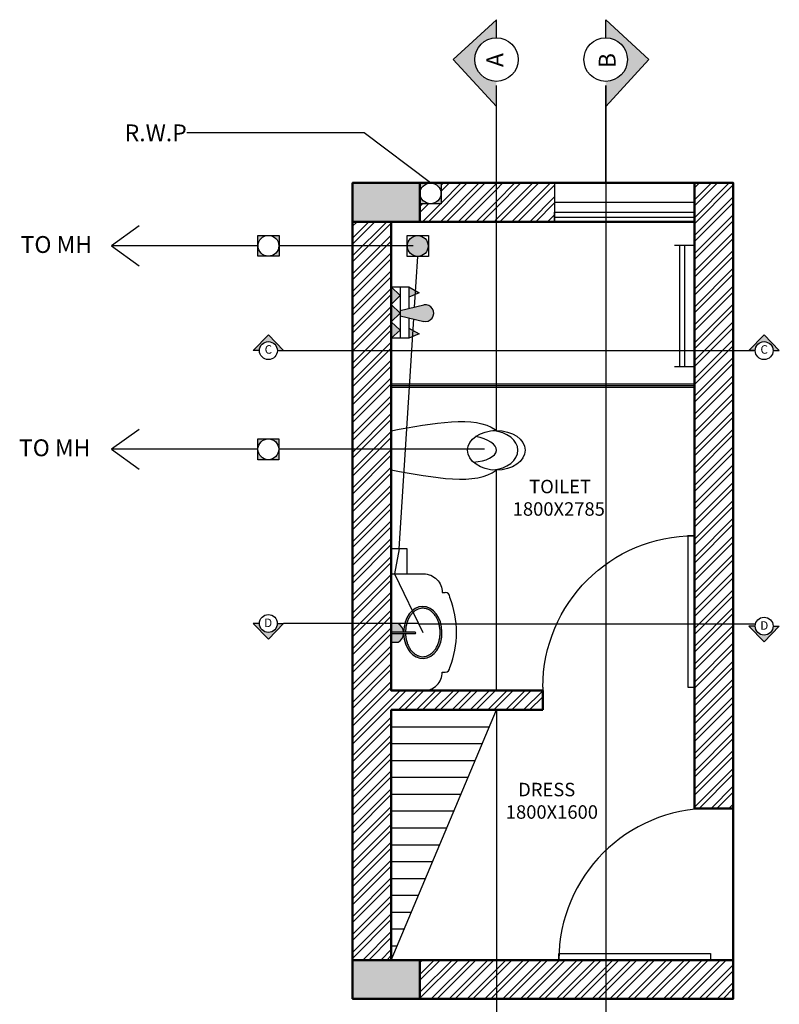
# Model space of a CAD drawing. Units: millimetres. Extents: x -2204 to 11247, y -2365 to 12631.
# Tile 2 of 3: x -2204 to 2305, y 2752 to 8600. Entities that reach past the tile are written whole.
import ezdxf
from ezdxf import colors
from ezdxf.entities.mleader import LeaderData, LeaderLine
from ezdxf.math import Vec2, Vec3

# ---------------------------------------------------------------- set-up
doc = ezdxf.new("R2010")
doc.units = ezdxf.units.MM
doc.header["$MEASUREMENT"] = 0
for name, color, linetype, lineweight in [('A-ANNO-SYMB', 2, 'Continuous', 25), ('A-ANNO-TEXT', 7, 'Continuous', 18), ('A-AREA-IDEN', 3, 'Continuous', 18), ('A-DOOR', 4, 'Continuous', 25), ('A-FLOR-FIXT', 8, 'Continuous', 25), ('A-FLOR-STRS', 3, 'Continuous', 25), ('A-GLAZ', 4, 'Continuous', 25), ('A-WALL', 7, 'Continuous', 50), ('A-WALL-PATT', 8, 'Continuous', 18), ('P-SANR', 5, 'Continuous', 25)]:
    doc.layers.add(name, color=color, linetype=linetype, lineweight=lineweight)
doc.styles.get("Standard").update_dxf_attribs({"font": 'arial.ttf'})

# ---------------------------------------------------------------- blocks, each defined once
blk = doc.blocks.new('*U2')
for p, q in [((0, 0), (0, -6)), ((40, 0), (40, -6))]:
    blk.add_line(p, q)
blk.add_lwpolyline([(0, 0), (0, 40), (1.75, 40), (1.75, 0)], close=True)
blk.add_arc((0, 0), 40, 0, 90)
blk = doc.blocks.new('SECT-MARK-AB')
for p, q in [((0, 407.4), (0, 515.4)), ((256.9, 278.3), (0, 515.4)), ((256.9, 278.3), (0, 0))]:
    blk.add_line(p, q)
blk = doc.blocks.new('SECT-MARK-CD')
for points in [[(36.9, 92.8), (0, 92.8), (90.1, 0)], [(143.4, 92.8), (180.2, 92.8), (90.1, 0)]]:
    blk.add_lwpolyline(points)
blk.add_circle((90.1, 92.8), 53.2)

msp = doc.modelspace()

# ---------------------------------------------------------------- hatches: boundary and pattern name
at = {"layer": 'A-ANNO-SYMB'}
h = msp.add_hatch(color=256, dxfattribs=at)
h.dxf.hatch_style = 1
h.paths.add_polyline_path([(369.3, 8362.8), (626.2, 8084.4), (626.2, 8233.7, -0.414214), (497.1, 8362.8, -0.414214), (626.2, 8491.8), (626.2, 8599.8)])
h = msp.add_hatch(color=256, dxfattribs=at)
h.dxf.hatch_style = 1
h.paths.add_polyline_path([(1531.6, 8362.8), (1274.8, 8084.4), (1274.8, 8233.7, 0.414214), (1403.8, 8362.8, 0.414214), (1274.8, 8491.8), (1274.8, 8599.8)])
h = msp.add_hatch(color=256, dxfattribs=at)
h.dxf.hatch_style = 1
h.paths.add_polyline_path([(-780.8, 6634.5), (-817.7, 6634.5), (-727.6, 6727.3), (-637.4, 6634.5), (-674.3, 6634.5, 1)])
h = msp.add_hatch(color=256, dxfattribs=at)
h.dxf.hatch_style = 1
h.paths.add_polyline_path([(2215.3, 6727.3), (2125.2, 6634.5), (2162.1, 6634.5, -1), (2268.6, 6634.5), (2305.4, 6634.5)])
h = msp.add_hatch(color=256, dxfattribs=at)
h.dxf.hatch_style = 1
h.paths.add_polyline_path([(-781, 5013.8), (-817.9, 5013.8), (-727.7, 4921), (-637.6, 5013.8), (-674.5, 5013.8, -1)])
h = msp.add_hatch(color=256, dxfattribs=at)
h.dxf.hatch_style = 1
h.paths.add_polyline_path([(2162.1, 4998.1), (2125.2, 4998.1), (2215.3, 4905.3), (2305.4, 4998.1), (2268.6, 4998.1, -1)])
at = {"layer": 'A-FLOR-FIXT'}
h = msp.add_hatch(color=256, dxfattribs=at)
h.dxf.hatch_style = 1
h.paths.add_polyline_path([(2.1, 6909), (2.1, 6805.1), (54.5, 6857.1)])
h.paths.add_polyline_path([(2.1, 7013), (2.1, 6909), (54.5, 6961)])
h = msp.add_hatch(color=256, dxfattribs=at)
h.dxf.hatch_style = 1
h.paths.add_polyline_path([(146.2, 6990.6), (106.9, 7013), (106.9, 6951.9), (144.8, 6967.9)])
h.paths.add_polyline_path([(146.2, 6990.6), (144.8, 6967.9), (168.4, 6977.9)])
h.paths.add_polyline_path([(131.3, 6754.6), (106.9, 6768.6), (106.9, 6707.4), (129, 6716.7)])
h.paths.add_polyline_path([(131.3, 6754.6), (129, 6716.7), (168.4, 6733.4)])
h = msp.add_hatch(color=256, dxfattribs=at)
h.dxf.hatch_style = 1
h.paths.add_polyline_path([(196.1, 6905.8), (54.5, 6872.8), (54.5, 6841.3), (196.1, 6808.3, 1.198102)])
h = msp.add_hatch(color=256, dxfattribs=at)
h.dxf.hatch_style = 1
h.paths.add_polyline_path([(54.5, 6755.1), (2.1, 6805.1), (2.1, 6707.4)])
h = msp.add_hatch(color=256, dxfattribs=at)
h.dxf.hatch_style = 1
edge = h.paths.add_edge_path()
edge.add_ellipse((189.1, 4960.4), major_axis=(0, 154.8), ratio=0.736024, start_angle=94.12154, end_angle=449.11704)
edge.add_line((75.2, 4962.2), (86.2, 4962.2))
edge.add_spline(control_points=[(86.2, 4962.2), (86.3, 4969.1), (86.7, 4975.9), (88.3, 4990.5), (89.7, 4998.3), (93.3, 5013.3), (95.5, 5020.6), (100.8, 5034.6), (103.9, 5041.2), (110.8, 5053.7), (114.5, 5059.6), (122.7, 5070.3), (127.1, 5075.2), (136.3, 5083.9), (141.1, 5087.7), (151, 5094.1), (156.2, 5096.8), (166.6, 5100.9), (171.9, 5102.4), (181.2, 5103.9), (185.1, 5104.2), (189.1, 5104.2)], knot_values=[0, 0, 0, 0, 0.140113, 0.140113, 0.302333, 0.302333, 0.464553, 0.464553, 0.626773, 0.626773, 0.788993, 0.788993, 0.951213, 0.951213, 1.113432, 1.113432, 1.275652, 1.275652, 1.437872, 1.437872, 1.558315, 1.558315, 1.558315, 1.558315], degree=3, periodic=0)
edge.add_spline(control_points=[(189.1, 5104.2), (192.2, 5104.2), (195.2, 5104), (203.7, 5102.9), (209.1, 5101.6), (219.9, 5097.8), (225.1, 5095.3), (235.4, 5089), (240.4, 5085.2), (249.9, 5076.5), (254.4, 5071.6), (262.9, 5060.8), (266.8, 5054.9), (273.9, 5042.2), (277, 5035.4), (282.5, 5021.1), (284.9, 5013.7), (288.6, 4998.3), (289.9, 4990.4), (291.7, 4974.4), (292.1, 4966.2), (291.9, 4950), (291.4, 4941.9), (289.2, 4925.9), (287.6, 4918.1), (283.6, 4902.9), (281.1, 4895.6), (275.3, 4881.6), (272, 4874.9), (264.6, 4862.5), (260.6, 4856.8), (251.9, 4846.4), (247.3, 4841.7), (237.6, 4833.4), (232.5, 4829.9), (222.2, 4824.1), (216.9, 4821.8), (206.1, 4818.4), (200.6, 4817.3), (189.8, 4816.4), (184.4, 4816.6), (173.8, 4818), (168.5, 4819.4), (158, 4823.2), (152.9, 4825.7), (142.8, 4831.9), (138, 4835.5), (128.7, 4844), (124.2, 4848.7), (115.9, 4859.2), (112.1, 4865), (105.1, 4877.3), (101.9, 4883.9), (96.4, 4897.7), (94, 4904.9), (90.2, 4919.8), (88.8, 4927.5), (87.1, 4940.9), (86.6, 4946.5), (86.4, 4952.2)], knot_values=[1.626715, 1.626715, 1.626715, 1.626715, 1.718936, 1.718936, 1.884955, 1.884955, 2.050974, 2.050974, 2.216993, 2.216993, 2.383012, 2.383012, 2.549031, 2.549031, 2.71505, 2.71505, 2.881069, 2.881069, 3.047088, 3.047088, 3.213108, 3.213108, 3.379127, 3.379127, 3.545146, 3.545146, 3.711165, 3.711165, 3.877184, 3.877184, 4.043203, 4.043203, 4.209222, 4.209222, 4.375241, 4.375241, 4.54126, 4.54126, 4.707279, 4.707279, 4.869499, 4.869499, 5.031719, 5.031719, 5.193939, 5.193939, 5.356159, 5.356159, 5.518379, 5.518379, 5.680599, 5.680599, 5.842818, 5.842818, 6.005038, 6.005038, 6.167258, 6.167258, 6.283185, 6.283185, 6.283185, 6.283185], degree=3, periodic=0)
edge.add_line((86.4, 4952.2), (75.3, 4952.2))
h = msp.add_hatch(color=256, dxfattribs=at)
h.dxf.hatch_style = 1
h.paths.add_polyline_path([(42.5, 5014.1), (2.1, 5014.1), (2.1, 4961.7), (75, 4962.2, 0.253551)])
h.paths.add_polyline_path([(74.9, 4952.2), (2.1, 4952.2), (2.1, 4902.1), (42.5, 4902.1, 0.245989)])
h.paths.add_polyline_path([(142.9, 4962.6), (2.1, 4961.7), (2.1, 4952.2), (74.9, 4952.2), (75.3, 4952.2), (143, 4952.2, 1.006847)])
at = {"layer": 'A-WALL-PATT'}
h = msp.add_hatch(color=256, dxfattribs=at)
h.dxf.hatch_style = 1
h.paths.add_polyline_path([(172.1, 7630.1), (-227.9, 7630.1), (-227.9, 7400.1), (172.1, 7400.1)])
h.paths.add_polyline_path([(172.1, 3015.1), (-227.9, 3015.1), (-227.9, 2785.1), (172.1, 2785.1)])
h = msp.add_hatch(dxfattribs=at)
h.set_pattern_fill('ANSI32', color=256, scale=200)
h.paths.add_polyline_path([(2.1, 7257), (-227.9, 7257), (-227.9, 6634.5), (2.1, 6634.5)])
h.paths.add_polyline_path([(2.1, 7400.1), (-227.9, 7400.1), (-227.9, 7257), (2.1, 7257)])
h.paths.add_polyline_path([(2032.1, 7630.1), (1802.1, 7630.1), (1802.1, 7400.1), (1802.1, 6634.5), (2032.1, 6634.5)])
h.paths.add_polyline_path([(2032.1, 6634.5), (1802.1, 6634.5), (1802.1, 5011.8), (2032.1, 5011.8)])
h.paths.add_polyline_path([(2032.1, 4845.1), (2032.1, 5011.8), (1802.1, 5011.8), (1802.1, 4635.1), (1802.1, 4500.1), (1802.1, 3915.1), (1878.7, 3915.1, -0.005089), (1897.1, 3915.3), (2032.1, 3915.3)])
h = msp.add_hatch(dxfattribs=at)
h.set_pattern_fill('ANSI32', color=256, scale=200)
h.paths.add_polyline_path([(626.2, 7630.1), (298, 7630.1), (298, 7506.6), (172.1, 7506.6), (172.1, 7400.1), (626.2, 7400.1)])
h = msp.add_hatch(dxfattribs=at)
h.set_pattern_fill('ANSI32', color=256, scale=200)
h.paths.add_polyline_path([(971, 7515.1), (971, 7630.1), (626.2, 7630.1), (626.2, 7400.1), (971, 7400.1), (971, 7457.6)])
h = msp.add_hatch(dxfattribs=at)
h.set_pattern_fill('ANSI32', color=256, scale=200)
h.paths.add_polyline_path([(901.9, 4615.1), (551.1, 4615.1), (2.1, 4615.1), (2.1, 5308.2), (2.1, 5457), (2.1, 6634.5), (-227.9, 6634.5), (-227.9, 4385.1), (-227.9, 3015.1), (2.1, 3015.1), (2.1, 4500.1), (901.9, 4500.1)])
h = msp.add_hatch(dxfattribs=at)
h.set_pattern_fill('ANSI32', color=256, scale=200)
h.paths.add_polyline_path([(1274.8, 3015.1), (996.9, 3015.1), (626.2, 3015.1), (626.2, 2785.1), (1274.8, 2785.1)])
h.paths.add_polyline_path([(626.2, 3015.1), (172.1, 3015.1), (172.1, 2785.1), (626.2, 2785.1)])
h.paths.add_polyline_path([(2032.1, 3015.1), (1897.1, 3015.1), (1274.8, 3015.1), (1274.8, 2785.1), (2032.1, 2785.1)])
at = {"layer": 'P-SANR'}
h = msp.add_hatch(color=256, dxfattribs=at)
h.dxf.hatch_style = 1
h.paths.add_polyline_path([(298, 7630.1), (235, 7630.1, -0.414214), (296.8, 7568.4, -0.414214), (235, 7506.6), (298, 7506.6)])
h.paths.add_polyline_path([(173.3, 7568.4, -0.414214), (235, 7630.1), (172.1, 7630.1), (172.1, 7506.6), (235, 7506.6, -0.414214)])
h = msp.add_hatch(color=256, dxfattribs=at)
h.dxf.hatch_style = 1
h.paths.add_polyline_path([(-664.5, 7318.7), (-727.4, 7318.7, -0.414214), (-665.7, 7257, -0.414214), (-727.4, 7195.2), (-664.5, 7195.2)])
h.paths.add_polyline_path([(-789.2, 7257, -0.414214), (-727.4, 7318.7), (-790.3, 7318.7), (-790.3, 7195.2), (-727.4, 7195.2, -0.414214)])
h = msp.add_hatch(color=256, dxfattribs=at)
h.dxf.hatch_style = 1
h.paths.add_polyline_path([(97.3, 7255.7, 1), (220.8, 7255.7, 1)])
h = msp.add_hatch(color=256, dxfattribs=at)
h.dxf.hatch_style = 1
h.paths.add_polyline_path([(-664.8, 6110.2), (-727.7, 6110.2, -0.414214), (-666, 6048.4, -0.414214), (-727.7, 5986.7), (-664.8, 5986.7)])
h.paths.add_polyline_path([(-789.5, 6048.4, -0.414214), (-727.7, 6110.2), (-790.7, 6110.2), (-790.7, 5986.7), (-727.7, 5986.7, -0.414214)])

# ---------------------------------------------------------------- linework, layer by layer
at = {"layer": 'A-ANNO-SYMB'}
for p, q in [((626.2, 6160.1), (626.2, 8209.7)), ((1274.8, 7630.1), (1274.8, 8209.7)), ((1274.8, 8209.7), (1274.8, 2578.2)), ((-817.7, 6634.5), (-727.6, 6727.3)), ((-637.4, 6634.5), (-727.6, 6727.3)), ((-780.8, 6634.5), (-817.7, 6634.5)), ((-674.3, 6634.5), (2162.1, 6634.5)), ((626.2, 4615.1), (626.2, 5924.9)), ((163.3, 5013.8), (-637.6, 5013.8)), ((163.3, 5011.8), (2162.1, 5011.8)), ((626.2, 4500.1), (626.2, 2584.7))]:
    msp.add_line(p, q, dxfattribs=at)
for points in [[(2162.1, 6634.5), (2125.2, 6634.5), (2215.3, 6727.3)], [(2268.6, 6634.5), (2305.4, 6634.5), (2215.3, 6727.3)]]:
    msp.add_lwpolyline(points, dxfattribs=at)
for centre, radius in [((626.2, 8362.8), 129.1), ((1274.8, 8362.8), 129.1), ((-727.6, 6634.5), 53.2), ((2215.3, 6634.5), 53.2)]:
    msp.add_circle(centre, radius, dxfattribs=at)
at = {"layer": 'A-FLOR-FIXT'}
for p, q in [((1802.1, 7258.8), (1683.3, 7258.8)), ((1712.7, 7258.8), (1712.7, 6537.5)), ((1742.7, 7258.8), (1742.7, 6537.5)), ((140, 6892.7), (159, 7193.9)), ((54.5, 6961), (2.1, 7013)), ((54.5, 6961), (2.1, 6909)), ((54.5, 7013), (54.5, 6707.4)), ((106.9, 7013), (168.4, 6977.9)), ((168.4, 6977.9), (106.9, 6951.9)), ((54.5, 6857.1), (2.1, 6909)), ((54.5, 6872.8), (196.1, 6905.8)), ((54.5, 6857.1), (2.1, 6805.1)), ((54.5, 6841.3), (196.1, 6808.3)), ((106.9, 6768.6), (168.4, 6733.4)), ((168.4, 6733.4), (106.9, 6707.4)), ((1802.1, 6537.5), (1683.3, 6537.5)), ((2.1, 6437.8), (1802.1, 6437.8)), ((2.1, 6427.8), (1802.1, 6427.8)), ((2.1, 6417.8), (1802.1, 6417.8)), ((304.2, 5198.2), (322.5, 5198.2)), ((350, 5167.6), (350, 5170.6)), ((143, 4962.6), (2.1, 4961.7)), ((75.3, 4952.2), (2.1, 4952.2)), ((304.2, 4725.2), (322.5, 4725.2))]:
    msp.add_line(p, q, dxfattribs=at)
for points in [[(106.9, 6829.1), (106.9, 6707.4), (2.1, 6707.4), (2.1, 7013), (106.9, 7013), (106.9, 6885)], [(2.1, 6707.4), (54.5, 6755.1), (2.1, 6805.1)], [(194.2, 4615.1), (2.1, 4615.1), (2.1, 5308.2)], [(42.5, 5014.1), (2.1, 5014.1), (2.1, 4902.1), (42.5, 4902.1)], [(143, 4952.2), (143, 4952.2), (75.3, 4952.2)]]:
    msp.add_lwpolyline(points, dxfattribs=at)
for points in [[(56.7, 6753.1), (56.7, 6753.1)], [(2.1, 5308.2), (97.1, 5308.2), (97.1, 5457), (2.1, 5457)]]:
    msp.add_lwpolyline(points, close=True, dxfattribs=at)
for points in [[(2.1, 5308.2), (194.2, 5308.2, -0.414214), (304.2, 5198.2)], [(2.1, 4615.1), (194.2, 4615.1, 0.414214), (304.2, 4725.2)]]:
    msp.add_lwpolyline(points, format="xyb", dxfattribs=at)
for centre, radius, start, end in [((204.9, 6857.1), 49.5, 254.09291, 100.29965), ((322.5, 5170.6), 27.5, 0, 90), ((-178.4, 4960.1), 567.7, 338.56485, 21.43515), ((10.9, 4958.1), 64.3, 3.62425, 60.53461), ((10.9, 4958.1), 64.3, 299.46539, 354.74434), ((143, 4957.4), 5.21, 270, 90), ((322.5, 4752.7), 27.5, 270, 0)]:
    msp.add_arc(centre, radius, start, end, dxfattribs=at)
msp.add_ellipse((626.2, 6042.5), major_axis=(170.9, 0), ratio=0.688339, dxfattribs=at)
for centre, major_axis, ratio, start_param, end_param in [((582.4, 6042.5), (170.9, 0), 0.688339, 4.840953, 7.725418), ((455.7, 6050), (170.5, -7.5), 0.456599, 4.929487, 7.59789), ((189.1, 4960.4), (0, 154.8), 0.736024, 1.623784, 7.842639)]:
    msp.add_ellipse(centre, major_axis=major_axis, ratio=ratio, start_param=start_param, end_param=end_param, dxfattribs=at)
for points, knots in [([(2.1, 6158.4), (251.7, 6204.9), (501.3, 6251.3), (618, 6164.9), (618, 6164.9), (618, 6164.9), (618, 6164.9), (618.3, 6164.6), (618.7, 6164.4), (619.1, 6164.1), (620.9, 6162.8), (622.7, 6161.4), (624.5, 6160.1)], [0, 0, 0, 0, 609.395671, 609.395671, 609.395671, 609.398707, 609.398707, 609.398707, 611.282085, 611.282085, 611.282085, 620.680386, 620.680386, 620.680386, 620.680386]), ([(189.1, 5104.2), (185.1, 5104.2), (181.2, 5103.9), (171.9, 5102.4), (166.6, 5100.9), (156.2, 5096.8), (151, 5094.1), (141.1, 5087.7), (136.3, 5083.9), (127.1, 5075.2), (122.7, 5070.3), (114.5, 5059.6), (110.8, 5053.7), (103.9, 5041.2), (100.8, 5034.6), (95.5, 5020.6), (93.3, 5013.3), (89.7, 4998.3), (88.3, 4990.5), (86.7, 4975.9), (86.3, 4969.1), (86.2, 4962.2)], [0, 0, 0, 0, 0.120443, 0.120443, 0.282663, 0.282663, 0.444883, 0.444883, 0.607102, 0.607102, 0.769322, 0.769322, 0.931542, 0.931542, 1.093762, 1.093762, 1.255982, 1.255982, 1.418202, 1.418202, 1.558315, 1.558315, 1.558315, 1.558315]), ([(86.4, 4952.2), (86.6, 4946.5), (87.1, 4940.9), (88.8, 4927.5), (90.2, 4919.8), (94, 4904.9), (96.4, 4897.7), (101.9, 4883.9), (105.1, 4877.3), (112.1, 4865), (115.9, 4859.2), (124.2, 4848.7), (128.7, 4844), (138, 4835.5), (142.8, 4831.9), (152.9, 4825.7), (158, 4823.2), (168.5, 4819.4), (173.8, 4818), (184.4, 4816.6), (189.8, 4816.4), (200.6, 4817.3), (206.1, 4818.4), (216.9, 4821.8), (222.2, 4824.1), (232.5, 4829.9), (237.6, 4833.4), (247.3, 4841.7), (251.9, 4846.4), (260.6, 4856.8), (264.6, 4862.5), (272, 4874.9), (275.3, 4881.6), (281.1, 4895.6), (283.6, 4902.9), (287.6, 4918.1), (289.2, 4925.9), (291.4, 4941.9), (291.9, 4950), (292.1, 4966.2), (291.7, 4974.4), (289.9, 4990.4), (288.6, 4998.3), (284.9, 5013.7), (282.5, 5021.1), (277, 5035.4), (273.9, 5042.2), (266.8, 5054.9), (262.9, 5060.8), (254.4, 5071.6), (249.9, 5076.5), (240.4, 5085.2), (235.4, 5089), (225.1, 5095.3), (219.9, 5097.8), (209.1, 5101.6), (203.7, 5102.9), (195.2, 5104), (192.2, 5104.2), (189.1, 5104.2)], [1.626715, 1.626715, 1.626715, 1.626715, 1.742642, 1.742642, 1.904862, 1.904862, 2.067082, 2.067082, 2.229301, 2.229301, 2.391521, 2.391521, 2.553741, 2.553741, 2.715961, 2.715961, 2.878181, 2.878181, 3.040401, 3.040401, 3.202621, 3.202621, 3.36864, 3.36864, 3.534659, 3.534659, 3.700678, 3.700678, 3.866697, 3.866697, 4.032716, 4.032716, 4.198735, 4.198735, 4.364754, 4.364754, 4.530773, 4.530773, 4.696792, 4.696792, 4.862812, 4.862812, 5.028831, 5.028831, 5.19485, 5.19485, 5.360869, 5.360869, 5.526888, 5.526888, 5.692907, 5.692907, 5.858926, 5.858926, 6.024945, 6.024945, 6.190964, 6.190964, 6.283185, 6.283185, 6.283185, 6.283185])]:
    msp.add_open_spline(points, degree=3, knots=knots, dxfattribs=at)
for points in [[(619, 6164.1), (619, 6164.1), (619, 6164.1), (619, 6164.1)], [(2.1, 5926.2), (256.5, 5878.8), (511, 5831.5), (624.6, 5924.9)]]:
    msp.add_open_spline(points, degree=3, dxfattribs=at)
at = {"layer": 'A-FLOR-STRS'}
msp.add_line((2.1, 3015.1), (626.2, 4500.1), dxfattribs=at)
for points in [[(2.1, 4400.1), (584.1, 4400.1)], [(2.1, 4300.1), (542.1, 4300.1)], [(2.1, 4200.1), (500.1, 4200.1)], [(2.1, 4100.1), (458.1, 4100.1)], [(2.1, 4000.1), (416, 4000.1)], [(2.1, 3900.1), (374, 3900.1)], [(2.1, 3800.1), (332, 3800.1)], [(2.1, 3700.1), (290, 3700.1)], [(2.1, 3600.1), (247.9, 3600.1)], [(2.1, 3500.1), (205.9, 3500.1)], [(2.1, 3400.1), (163.9, 3400.1)], [(2.1, 3300.1), (121.9, 3300.1)], [(2.1, 3200.1), (79.8, 3200.1)], [(2.1, 3100.1), (37.8, 3100.1)]]:
    msp.add_lwpolyline(points, dxfattribs=at)
at = {"layer": 'A-GLAZ'}
for p, q in [((971, 7630.1), (971, 7400.1)), ((971, 7515.1), (1802.1, 7515.1)), ((971, 7515.1), (971, 7400.1)), ((971, 7400.1), (971, 7457.6)), ((971, 7457.6), (1802.1, 7457.6)), ((971, 7427.6), (1802.1, 7427.6))]:
    msp.add_line(p, q, dxfattribs=at)
at = {"layer": 'A-WALL'}
for p, q in [((1802.1, 7400.1), (1802.1, 7630.1)), ((902.1, 4615.1), (902.1, 4500.1)), ((1802.1, 3915.1), (2032.1, 3915.1)), ((1802.1, 3015.1), (2032.1, 3015.1)), ((626.2, 2785.1), (1274.8, 2785.1))]:
    msp.add_line(p, q, dxfattribs=at)
for points in [[(2032.1, 4385.1), (2032.1, 7630.1), (-227.9, 7630.1), (-227.9, 4385.1)], [(1802.1, 4615.1), (1802.1, 7400.1), (2.1, 7400.1), (2.1, 4615.1), (902.1, 4615.1)], [(2032.1, 4845.1), (2032.1, 2785.1), (-227.9, 2785.1), (-227.9, 4845.1)], [(551.1, 4615.1), (902.1, 4615.1)], [(1802.1, 4615.1), (1802.1, 3915.1)], [(2.1, 4500.1), (902.1, 4500.1)], [(1802.1, 3015.1), (2.1, 3015.1), (2.1, 4500.1)]]:
    msp.add_lwpolyline(points, dxfattribs=at)
for points in [[(-227.9, 7630.1), (172.1, 7630.1), (172.1, 7400.1), (-227.9, 7400.1)], [(-227.9, 3015.1), (172.1, 3015.1), (172.1, 2785.1), (-227.9, 2785.1)]]:
    msp.add_lwpolyline(points, close=True, dxfattribs=at)
at = {"layer": 'P-SANR'}
for p, q in [((-790.3, 7257), (-1659.3, 7257)), ((132.7, 7257), (-664.5, 7257)), ((49.6, 5457), (135.6, 6822.4)), ((-789.5, 6048.4), (-1659.3, 6048.4)), ((554.7, 6048.4), (-666, 6048.4)), ((49.6, 5457), (20.9, 5308.2)), ((20.9, 5308.2), (189.1, 4960.4))]:
    msp.add_line(p, q, dxfattribs=at)
for points in [[(172.1, 7630.1), (298, 7630.1), (298, 7506.6), (172.1, 7506.6)], [(-790.3, 7318.7), (-664.5, 7318.7), (-664.5, 7195.2), (-790.3, 7195.2)], [(96.1, 7317.4), (221.9, 7317.4), (221.9, 7193.9), (96.1, 7193.9)], [(-790.7, 6110.2), (-664.8, 6110.2), (-664.8, 5986.7), (-790.7, 5986.7)]]:
    msp.add_lwpolyline(points, close=True, dxfattribs=at)
for points in [[(-1495, 7375), (-1659.3, 7257), (-1495, 7138.9)], [(-1495, 6166.5), (-1659.3, 6048.4), (-1495, 5930.3)]]:
    msp.add_lwpolyline(points, dxfattribs=at)
for centre in [(235, 7568.4), (-727.4, 7257), (159, 7255.7), (-727.7, 6048.4)]:
    msp.add_circle(centre, 61.7, dxfattribs=at)

# ---------------------------------------------------------------- block references
at = {"layer": 'A-ANNO-SYMB', "extrusion": (0, 0, -1), "zscale": -1}
msp.add_blockref('SECT-MARK-AB', (-626.2, 8084.4), dxfattribs=at)
at = {"layer": 'A-ANNO-SYMB'}
for name, p in [('SECT-MARK-AB', (1274.8, 8084.4)), ('SECT-MARK-CD', (-817.9, 4921)), ('SECT-MARK-CD', (2125.2, 4905.3))]:
    msp.add_blockref(name, p, dxfattribs=at)
at = {"layer": 'A-DOOR', "xscale": -22.50466275476805, "yscale": 22.50466275476805, "zscale": 22.50466275476805}
msp.add_blockref('*U2', (1802.1, 4635.1), dxfattribs=at)
at = {"layer": 'A-DOOR', "xscale": 22.50466275476805, "yscale": 22.50466275476805, "zscale": 22.50466275476805, "rotation": 90}
msp.add_blockref('*U2', (1897.1, 3015.1), dxfattribs=at)

# ---------------------------------------------------------------- texts
at = {"layer": 'A-ANNO-SYMB', "char_height": 100, "rotation": 90}
for s, insert, attachment_point in [('A', (667.2, 8401.7), 9), ('B', (1233.7, 8401.7), 3)]:
    msp.add_mtext_dynamic_manual_height_columns(s, width=142.124, gutter_width=1, heights=[0], dxfattribs=dict(at, insert=insert, attachment_point=attachment_point))
at = {"layer": 'A-ANNO-SYMB', "char_height": 50.6}
for s, insert, attachment_point in [('C', (-705.7, 6666.6), 3), ('C', (2193.5, 6666.6), 1), ('D', (-705.1, 5042.8), 3), ('D', (2192.7, 5027.1), 1)]:
    msp.add_mtext_dynamic_manual_height_columns(s, width=71.968, gutter_width=0.506, heights=[0], dxfattribs=dict(at, insert=insert, attachment_point=attachment_point))
at = {"layer": 'A-ANNO-TEXT', "char_height": 100, "attachment_point": 1}
for insert in [(-2198.5, 7314.6), (-2208.2, 6107.2)]:
    msp.add_mtext_dynamic_manual_height_columns('TO MH ', width=820.155, gutter_width=1, heights=[0], dxfattribs=dict(at, insert=insert))
at = {"layer": 'A-AREA-IDEN', "char_height": 100, "attachment_point": 1}
for s, insert in [('{\\H0.8x;    TOILET\\P1800X2785}', (722.8, 5867.1)), ('{\\H0.8x;   DRESS\\P1800X1600}', (681.9, 4067.4))]:
    msp.add_mtext_dynamic_manual_height_columns(s, width=820.155, gutter_width=1, heights=[0], dxfattribs=dict(at, insert=insert))

# ---------------------------------------------------------------- leaders
at = {"layer": 'A-ANNO-TEXT'}
ml = msp.add_multileader_mtext('Standard', dxfattribs=at)
ml.set_content('R.W.P ', color=256)
ml.set_leader_properties()
ml.build(insert=Vec2(0, 0))
ml.multileader.update_dxf_attribs({"dogleg_length": 0.36, "arrow_head_size": 0.18})
ctx = ml.context
ctx.base_point, ctx.char_height, ctx.arrow_head_size, ctx.landing_gap_size, ctx.plane_origin = Vec3(-1598.7, 7927.7), 100, 0.18, 0.09, Vec3(235, 7630.1)
ctx.text_align_type = 2
notes = []
notes.append((ctx, [(0, (1, 1, 0), (-159.5, 7927.7), (-1, 0), 1052.5, [(0, [(235, 7630.1)], 0, [])])]))
ctx.mtext.insert, ctx.mtext.alignment, ctx.mtext.flow_direction = Vec3(-1212.2, 7977.7), 3, 5
for ctx, leaders in notes:
    for number, flags, end, landing, length, lines in leaders:
        leader = LeaderData()
        leader.index, (leader.has_last_leader_line, leader.has_dogleg_vector, leader.attachment_direction) = number, flags
        leader.last_leader_point, leader.dogleg_vector, leader.dogleg_length = Vec3(end), Vec3(landing), length
        for number, points, colour, breaks in lines:
            line = LeaderLine()
            line.index, line.vertices, line.color, line.breaks = number, Vec3.list(points), colors.encode_raw_color(colour), breaks
            leader.lines.append(line)
        ctx.leaders.append(leader)

doc.saveas('drawing.dxf')
